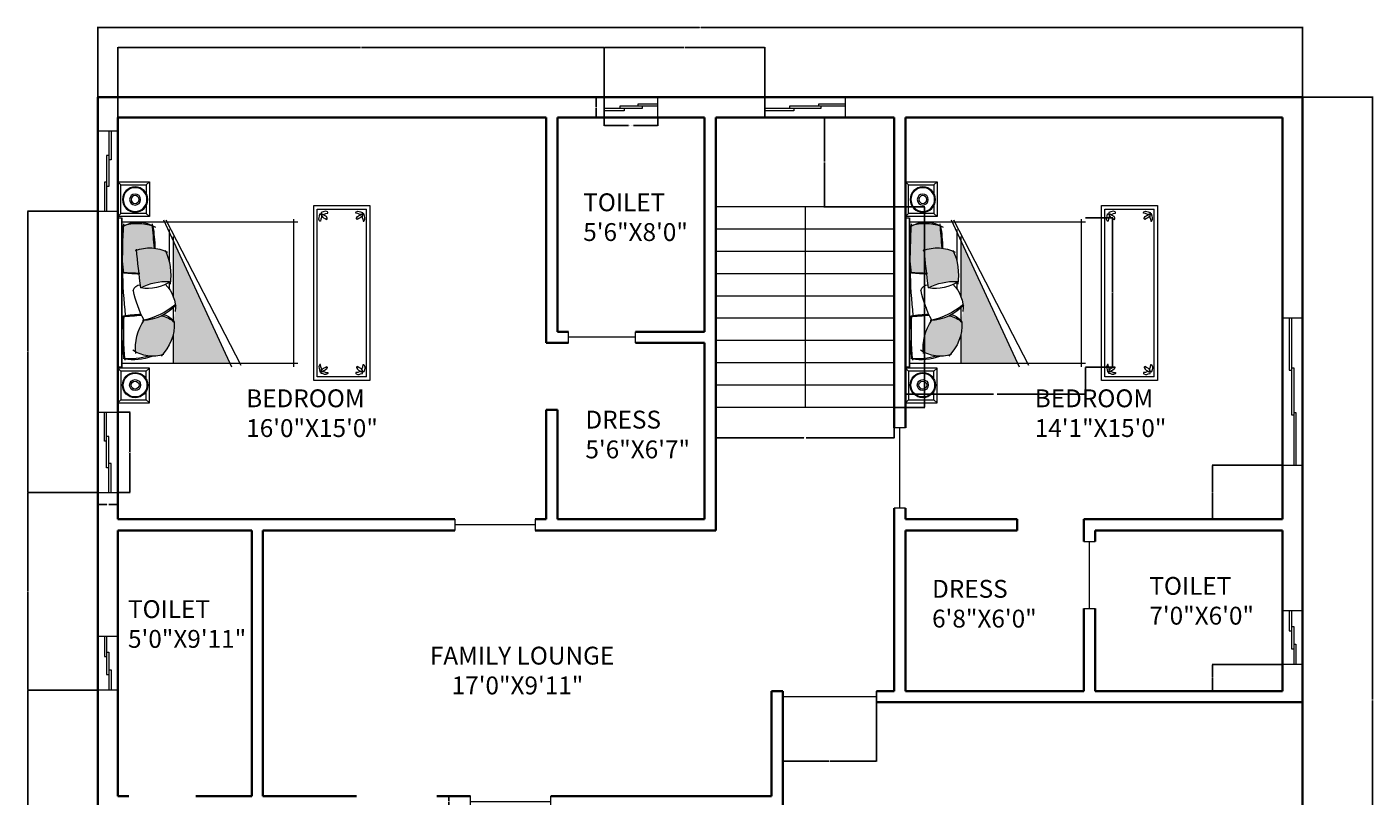
# Model space of a CAD drawing. Units: inches. Extents: x 1569 to 2779, y 1228 to 1844.
# Tile 6 of 6: x 2176 to 2779, y 1500 to 1844. Entities that reach past the tile are written whole.
import ezdxf

# ---------------------------------------------------------------- set-up
doc = ezdxf.new("R2010")
doc.units = ezdxf.units.IN
for name, color, linetype, lineweight in [('0.10', 252, 'Continuous', 9), ('0.15', 34, 'Continuous', 15), ('A-ANNO-DIMS', 2, 'Continuous', 18), ('A-AREA-IDEN', 7, 'Continuous', 18), ('A-DOOR', 3, 'Continuous', 20), ('A-FLOR-STRS', 4, 'Continuous', 18), ('A-FURN', 8, 'Continuous', 13), ('A-FURN-PATT', 116, 'Continuous', 9), ('A-GLAZ', 5, 'Continuous', 18), ('A-WALL', 7, 'Continuous', 35)]:
    doc.layers.add(name, color=color, linetype=linetype, lineweight=lineweight)
doc.styles.get("Standard").update_dxf_attribs({"font": 'arial.ttf'})
doc.dimstyles.get("Standard").update_dxf_attribs({"dimtxt": 0.18, "dimasz": 0.18, "dimexe": 0.18, "dimexo": 0.0625, "dimgap": 0.09, "dimtad": 0, "dimtih": 1, "dimtoh": 1, "dimdec": 4, "dimzin": 0, "dimdsep": 46, "dimtxsty": 'Standard', "dimcen": 0.09, "dimadec": 0, "dimazin": 0, "dimtfac": 1, "dimtdec": 4, "dimtofl": 0, "dimtmove": 0, "dimatfit": 3, "dimfxl": 1, "dimtolj": 1, "dimtzin": 0, "dimarcsym": 0})

# ---------------------------------------------------------------- blocks, each defined once
blk = doc.blocks.new('camita')
at = {"layer": '0.10'}
for p, q in [((-0.85, -0.045), (0.85, -0.045)), ((-0.805, -0.045), (-0.805, -2.048)), ((0.805, -0.045), (0.805, -2.048)), ((-0.827, -0.521), (0.846, -1.293)), ((-0.827, -0.548), (0.824, -1.399)), ((-0.716, -0.585), (-0.355, -0.585)), ((-0.114, -0.585), (-0.049, -0.585)), ((-0.638, -0.63), (0.043, -0.63)), ((0.175, -0.63), (0.318, -0.63)), ((0.474, -0.63), (0.805, -0.63)), ((-0.835, -2), (0.846, -2))]:
    blk.add_line(p, q, dxfattribs=at)
blk.add_lwpolyline([(-0.85, -0.041), (0.85, -0.041), (0.85, 0), (-0.85, 0)], close=True, dxfattribs=at)
for centre, radius, start, end in [((-0.457, -0.236), 0.344, 147.51, 213.8336), ((-0.2, -0.227), 0.586, 163.9263, 197.1409), ((-0.364, -5.846), 5.791, 83.8073, 94.1211), ((-0.51, -1.723), 1.678, 80.1255, 98.6619), ((2.353, -0.053), 2.58, 180.1063, 184.3854), ((-1.544, -0.245), 1.333, 359.9394, 7.5533), ((1.581, -0.289), 1.335, 170.3802, 178.9914), ((-1.44, -0.061), 1.712, 352.9291, 0.3959), ((0.452, -3.067), 3, 83.9026, 93.6759), ((0.486, -1.629), 1.578, 80.1602, 98.06), ((0.029, -0.138), 0.726, 342.5841, 6.0048), ((0.133, -0.17), 0.631, 339.923, 8.7433), ((-0.054, -0.363), 0.454, 159.3026, 206.5026), ((-1.33, -9.675), 9.499, 82.2708, 84.9399), ((0.458, -0.545), 0.584, 151.0456, 184.1497), ((-0.534, -0.339), 0.487, 327.2644, 9.0473), ((-0.007, -0.258), 0.0828, 100.018, 179.736), ((-0.293, -1.438), 1.29, 61.9749, 77.8435), ((-0.199, -0.274), 0.516, 310.7395, 359.0576), ((-0.567, -0.087), 0.906, 321.6953, 346.4626), ((0.627, -0.752), 0.551, 82.9691, 124.6739), ((0.32, -0.394), 0.404, 341.4524, 33.4512), ((-1.867, -14.986), 14.632, 84.6597, 85.7516), ((-0.46, 1.486), 1.909, 260.953, 268.6517), ((-0.2, 0.064), 0.667, 244.7809, 279.0606), ((0.179, -0.272), 0.383, 224.5284, 275.2229), ((0.438, -0.483), 0.19, 193.6849, 236.7035), ((0.571, -0.432), 0.315, 192.9388, 221.9636), ((0.361, -0.133), 0.51, 267.2589, 315.2997)]:
    blk.add_arc(centre, radius, start, end, dxfattribs=at)
blk = doc.blocks.new('VELADOR')
at = {"layer": '0.15'}
for p, q in [((-0.248, 0), (-0.203, -0.045)), ((0.248, 0), (0.202, -0.045)), ((-0.203, -0.405), (-0.248, -0.45)), ((0.248, -0.45), (0.202, -0.405))]:
    blk.add_line(p, q, dxfattribs=at)
blk.add_lwpolyline([(-0.248, 0), (-0.248, -0.45), (0.248, -0.45), (0.248, 0)], close=True, dxfattribs=at)
blk.add_lwpolyline([(0.092, -0.405), (0.202, -0.405), (0.202, -0.045), (-0.203, -0.045), (-0.203, -0.405), (-0.082, -0.405)], dxfattribs=at)
for radius in [0.18, 0.169, 0.0788, 0.0563]:
    blk.add_circle((0.005, -0.247), radius, dxfattribs=at)
blk = doc.blocks.new('carpet-7')
at = {"color": 0, "linetype": 'ByBlock'}
for p, q in [((-1.022, 0), (0, 0)), ((0, 0), (0, -0.54)), ((-1.694, -0.54), (-1.694, 0)), ((-1.694, 0), (-1.022, 0)), ((-1.658, -0.508), (-1.658, -0.032)), ((-1.658, -0.032), (-0.036, -0.032)), ((-1.636, -0.116), (-1.634, -0.103)), ((-1.629, -0.131), (-1.636, -0.116)), ((-1.634, -0.103), (-1.63, -0.09)), ((-1.63, -0.09), (-1.626, -0.07)), ((-1.626, -0.07), (-1.617, -0.069)), ((-1.617, -0.069), (-1.612, -0.072)), ((-1.615, -0.116), (-1.617, -0.134)), ((-1.608, -0.102), (-1.615, -0.116)), ((-1.611, -0.056), (-1.612, -0.064)), ((-1.612, -0.064), (-1.609, -0.068)), ((-1.612, -0.072), (-1.606, -0.089)), ((-1.59, -0.052), (-1.611, -0.056)), ((-1.609, -0.068), (-1.591, -0.073)), ((-1.609, -0.079), (-1.603, -0.072)), ((-1.599, -0.096), (-1.609, -0.079)), ((-1.606, -0.089), (-1.608, -0.102)), ((-1.603, -0.072), (-1.597, -0.072)), ((-1.593, -0.108), (-1.599, -0.096)), ((-1.597, -0.072), (-1.581, -0.081)), ((-1.585, -0.12), (-1.593, -0.108)), ((-1.591, -0.073), (-1.576, -0.072)), ((-1.575, -0.049), (-1.59, -0.052)), ((-1.569, -0.127), (-1.585, -0.12)), ((-1.581, -0.081), (-1.573, -0.092)), ((-1.576, -0.072), (-1.561, -0.066)), ((-1.561, -0.046), (-1.575, -0.049)), ((-1.573, -0.092), (-1.568, -0.107)), ((-1.563, -0.127), (-1.569, -0.127)), ((-1.568, -0.107), (-1.557, -0.123)), ((-1.557, -0.123), (-1.563, -0.127)), ((-1.544, -0.053), (-1.561, -0.046)), ((-1.561, -0.066), (-1.54, -0.064)), ((-1.54, -0.056), (-1.544, -0.053)), ((-1.54, -0.064), (-1.54, -0.056)), ((-0.151, -0.056), (-0.148, -0.053)), ((-0.151, -0.064), (-0.151, -0.056)), ((-0.131, -0.066), (-0.151, -0.064)), ((-0.148, -0.053), (-0.131, -0.046)), ((-0.124, -0.107), (-0.134, -0.123)), ((-0.134, -0.123), (-0.128, -0.127)), ((-0.131, -0.046), (-0.116, -0.049)), ((-0.115, -0.072), (-0.131, -0.066)), ((-0.128, -0.127), (-0.122, -0.127)), ((-0.119, -0.092), (-0.124, -0.107)), ((-0.122, -0.127), (-0.107, -0.12)), ((-0.11, -0.081), (-0.119, -0.092)), ((-0.116, -0.049), (-0.102, -0.052)), ((-0.101, -0.073), (-0.115, -0.072)), ((-0.095, -0.072), (-0.11, -0.081)), ((-0.107, -0.12), (-0.098, -0.108)), ((-0.102, -0.052), (-0.08, -0.056)), ((-0.083, -0.068), (-0.101, -0.073)), ((-0.098, -0.108), (-0.092, -0.096)), ((-0.089, -0.072), (-0.095, -0.072)), ((-0.092, -0.096), (-0.083, -0.079)), ((-0.083, -0.079), (-0.089, -0.072)), ((-0.079, -0.072), (-0.085, -0.089)), ((-0.085, -0.089), (-0.084, -0.102)), ((-0.084, -0.102), (-0.077, -0.116)), ((-0.079, -0.064), (-0.083, -0.068)), ((-0.08, -0.056), (-0.079, -0.064)), ((-0.074, -0.069), (-0.079, -0.072)), ((-0.077, -0.116), (-0.074, -0.134)), ((-0.066, -0.07), (-0.074, -0.069)), ((-0.061, -0.09), (-0.066, -0.07)), ((-0.062, -0.131), (-0.055, -0.116)), ((-0.058, -0.103), (-0.061, -0.09)), ((-0.055, -0.116), (-0.058, -0.103)), ((-0.036, -0.032), (-0.036, -0.508)), ((-1.626, -0.134), (-1.629, -0.131)), ((-1.617, -0.134), (-1.626, -0.134)), ((-0.074, -0.134), (-0.066, -0.134)), ((-0.066, -0.134), (-0.062, -0.131)), ((-1.658, -0.508), (-0.036, -0.508)), ((-1.629, -0.409), (-1.636, -0.424)), ((-1.636, -0.424), (-1.634, -0.437)), ((-1.634, -0.437), (-1.63, -0.45)), ((-1.63, -0.45), (-1.626, -0.47)), ((-1.626, -0.406), (-1.629, -0.409)), ((-1.617, -0.406), (-1.626, -0.406)), ((-1.626, -0.47), (-1.617, -0.471)), ((-1.615, -0.424), (-1.617, -0.406)), ((-1.617, -0.471), (-1.612, -0.468)), ((-1.608, -0.438), (-1.615, -0.424)), ((-1.612, -0.468), (-1.606, -0.451)), ((-1.612, -0.476), (-1.609, -0.472)), ((-1.611, -0.484), (-1.612, -0.476)), ((-1.59, -0.488), (-1.611, -0.484)), ((-1.599, -0.444), (-1.609, -0.461)), ((-1.609, -0.461), (-1.603, -0.468)), ((-1.609, -0.472), (-1.591, -0.467)), ((-1.606, -0.451), (-1.608, -0.438)), ((-1.603, -0.468), (-1.597, -0.468)), ((-1.593, -0.432), (-1.599, -0.444)), ((-1.597, -0.468), (-1.581, -0.459)), ((-1.585, -0.42), (-1.593, -0.432)), ((-1.591, -0.467), (-1.576, -0.468)), ((-1.575, -0.491), (-1.59, -0.488)), ((-1.569, -0.413), (-1.585, -0.42)), ((-1.581, -0.459), (-1.573, -0.448)), ((-1.576, -0.468), (-1.561, -0.474)), ((-1.561, -0.494), (-1.575, -0.491)), ((-1.573, -0.448), (-1.568, -0.433)), ((-1.563, -0.413), (-1.569, -0.413)), ((-1.568, -0.433), (-1.557, -0.417)), ((-1.557, -0.417), (-1.563, -0.413)), ((-1.561, -0.474), (-1.54, -0.476)), ((-1.544, -0.487), (-1.561, -0.494)), ((-1.54, -0.484), (-1.544, -0.487)), ((-1.54, -0.476), (-1.54, -0.484)), ((-0.131, -0.474), (-0.151, -0.476)), ((-0.151, -0.476), (-0.151, -0.484)), ((-0.151, -0.484), (-0.148, -0.487)), ((-0.148, -0.487), (-0.131, -0.494)), ((-0.134, -0.417), (-0.128, -0.413)), ((-0.124, -0.433), (-0.134, -0.417)), ((-0.115, -0.468), (-0.131, -0.474)), ((-0.131, -0.494), (-0.116, -0.491)), ((-0.128, -0.413), (-0.122, -0.413)), ((-0.119, -0.448), (-0.124, -0.433)), ((-0.122, -0.413), (-0.107, -0.42)), ((-0.11, -0.459), (-0.119, -0.448)), ((-0.116, -0.491), (-0.102, -0.488)), ((-0.101, -0.467), (-0.115, -0.468)), ((-0.095, -0.468), (-0.11, -0.459)), ((-0.107, -0.42), (-0.098, -0.432)), ((-0.102, -0.488), (-0.08, -0.484)), ((-0.083, -0.472), (-0.101, -0.467)), ((-0.098, -0.432), (-0.092, -0.444)), ((-0.089, -0.468), (-0.095, -0.468)), ((-0.092, -0.444), (-0.083, -0.461)), ((-0.083, -0.461), (-0.089, -0.468)), ((-0.085, -0.451), (-0.084, -0.438)), ((-0.079, -0.468), (-0.085, -0.451)), ((-0.084, -0.438), (-0.077, -0.424)), ((-0.079, -0.476), (-0.083, -0.472)), ((-0.08, -0.484), (-0.079, -0.476)), ((-0.074, -0.471), (-0.079, -0.468)), ((-0.077, -0.424), (-0.074, -0.406)), ((-0.074, -0.406), (-0.066, -0.406)), ((-0.066, -0.47), (-0.074, -0.471)), ((-0.066, -0.406), (-0.062, -0.409)), ((-0.061, -0.45), (-0.066, -0.47)), ((-0.062, -0.409), (-0.055, -0.424)), ((-0.058, -0.437), (-0.061, -0.45)), ((-0.055, -0.424), (-0.058, -0.437)), ((0, -0.54), (-1.694, -0.54))]:
    blk.add_line(p, q, dxfattribs=at)
blk = doc.blocks.new('WIN-24IN')
for p, q in [((9, 24), (0, 24)), ((3, 24), (3, 15)), ((4, 24), (4, 7)), ((3, 15), (4, 15)), ((4, 17), (5, 17)), ((5, 17), (5, 0)), ((4, 7), (5, 7)), ((5, 9), (6, 9)), ((6, 9), (6, 0)), ((9, 0), (0, 0))]:
    blk.add_line(p, q)
blk = doc.blocks.new('WIN-66IN')
for p, q in [((0, 0), (0, 9)), ((66, 0), (66, 9)), ((0, 4), (43.5, 4)), ((0, 3), (23.5, 3)), ((22.5, 5), (66, 5)), ((22.5, 4), (22.5, 5)), ((23.5, 3), (23.5, 4)), ((42.5, 6), (66, 6)), ((42.5, 5), (42.5, 6)), ((43.5, 4), (43.5, 5))]:
    blk.add_line(p, q)
blk = doc.blocks.new('WIN-36IN-A')
for p, q in [((0, 9), (0, 0)), ((36, 9), (36, 0)), ((25, 4), (0, 4)), ((13, 3), (0, 3)), ((36, 5), (11, 5)), ((11, 5), (11, 4)), ((13, 4), (13, 3)), ((24, 6), (24, 5)), ((36, 6), (24, 6)), ((25, 5), (25, 4))]:
    blk.add_line(p, q)
blk = doc.blocks.new('WIN-36IN-B')
for p, q in [((0, 36), (9, 36)), ((3, 23), (3, 36)), ((4, 11), (4, 36)), ((5, 25), (4, 25)), ((5, 0), (5, 25)), ((4, 23), (3, 23)), ((6, 13), (5, 13)), ((6, 0), (6, 13)), ((5, 11), (4, 11)), ((0, 0), (9, 0))]:
    blk.add_line(p, q)
blk = doc.blocks.new('DOOR-30IN')
for p, q in [((0, 5), (0, 0)), ((0, 2.5), (30, 2.5)), ((30, 5), (30, 0))]:
    blk.add_line(p, q)
blk = doc.blocks.new('DOOR-36IN')
for p, q in [((0, 5), (0, 0)), ((36, 2.5), (0, 2.5)), ((36, 5), (36, 0))]:
    blk.add_line(p, q)
blk = doc.blocks.new('STAIR-RETURN-FLIGHT')
for p, q in [((80, 90), (0, 90)), ((40, 90), (40, 0)), ((80, 80), (0, 80)), ((80, 70), (0, 70)), ((80, 60), (0, 60)), ((80, 50), (0, 50)), ((80, 40), (0, 40)), ((80, 30), (0, 30)), ((80, 20), (0, 20)), ((80, 10), (0, 10)), ((80, 0), (0, 0))]:
    blk.add_line(p, q)
blk = doc.blocks.new('*D22')
at = {"layer": 'A-ANNO-DIMS', "color": 0, "lineweight": -2, "transparency": 16777216}
for p, q in [((2359.41, 1499.88), (2364.93, 1499.88)), ((2364.75, 1499.7), (2364.75, 1497.56)), ((2364.75, 1495.06), (2364.75, 1497.2)), ((2359.41, 1494.88), (2364.93, 1494.88))]:
    blk.add_line(p, q, dxfattribs=at)
at = {"layer": 'A-ANNO-DIMS', "color": 0, "transparency": 16777216}
for points in [[(2364.72, 1499.7), (2364.78, 1499.7), (2364.75, 1499.88)], [(2364.72, 1495.06), (2364.78, 1495.06), (2364.75, 1494.88)]]:
    blk.add_solid(points, dxfattribs=at)
at = {"layer": 'Defpoints', "color": 0, "transparency": 16777216}
for p in [(2359.35, 1499.88), (2364.75, 1499.88), (2359.35, 1494.88)]:
    blk.add_point(p, dxfattribs=at)
at = {"layer": 'A-ANNO-DIMS', "color": 0, "transparency": 16777216, "insert": (2364.75, 1497.38), "char_height": 0.18, "attachment_point": 5}
blk.add_mtext('\\A1;5 TYP.', dxfattribs=at)
blk = doc.blocks.new('*D23')
at = {"layer": 'A-ANNO-DIMS', "color": 0, "lineweight": -2, "transparency": 16777216}
for p, q in [((2434.35, 1803.82), (2434.35, 1800.1)), ((2458.35, 1803.82), (2458.35, 1800.1)), ((2434.53, 1800.28), (2445.23, 1800.28)), ((2458.17, 1800.28), (2447.47, 1800.28))]:
    blk.add_line(p, q, dxfattribs=at)
at = {"layer": 'A-ANNO-DIMS', "color": 0, "transparency": 16777216}
for points in [[(2434.53, 1800.31), (2434.53, 1800.25), (2434.35, 1800.28)], [(2458.17, 1800.31), (2458.17, 1800.25), (2458.35, 1800.28)]]:
    blk.add_solid(points, dxfattribs=at)
at = {"layer": 'Defpoints', "color": 0, "transparency": 16777216}
for p in [(2434.35, 1803.88), (2458.35, 1803.88), (2458.35, 1800.28)]:
    blk.add_point(p, dxfattribs=at)
at = {"layer": 'A-ANNO-DIMS', "color": 0, "transparency": 16777216, "insert": (2446.35, 1800.28), "char_height": 0.18, "attachment_point": 5}
blk.add_mtext('\\A1;WINDOW 24 TYP.', dxfattribs=at)
blk = doc.blocks.new('*D24')
at = {"layer": 'A-ANNO-DIMS', "color": 0, "lineweight": -2, "transparency": 16777216}
for p, q in [((2434.29, 1812.88), (2430.57, 1812.88)), ((2430.75, 1812.7), (2430.75, 1808.56)), ((2434.29, 1803.88), (2430.57, 1803.88)), ((2430.75, 1804.06), (2430.75, 1808.2))]:
    blk.add_line(p, q, dxfattribs=at)
at = {"layer": 'A-ANNO-DIMS', "color": 0, "transparency": 16777216}
for points in [[(2430.72, 1812.7), (2430.78, 1812.7), (2430.75, 1812.88)], [(2430.72, 1804.06), (2430.78, 1804.06), (2430.75, 1803.88)]]:
    blk.add_solid(points, dxfattribs=at)
at = {"layer": 'Defpoints', "color": 0, "transparency": 16777216}
for p in [(2434.35, 1812.88), (2430.75, 1803.88), (2434.35, 1803.88)]:
    blk.add_point(p, dxfattribs=at)
at = {"layer": 'A-ANNO-DIMS', "color": 0, "transparency": 16777216, "insert": (2430.75, 1808.38), "char_height": 0.18, "attachment_point": 5}
blk.add_mtext('\\A1;9 TYP.', dxfattribs=at)
blk = doc.blocks.new('*D27')
at = {"layer": 'A-ANNO-DIMS', "color": 0, "lineweight": -2, "transparency": 16777216}
for p, q in [((2216.41, 1671.88), (2221.93, 1671.88)), ((2221.75, 1671.7), (2221.75, 1654.06)), ((2221.75, 1636.06), (2221.75, 1653.7)), ((2216.41, 1635.88), (2221.93, 1635.88))]:
    blk.add_line(p, q, dxfattribs=at)
at = {"layer": 'A-ANNO-DIMS', "color": 0, "transparency": 16777216}
for points in [[(2221.72, 1671.7), (2221.78, 1671.7), (2221.75, 1671.88)], [(2221.72, 1636.06), (2221.78, 1636.06), (2221.75, 1635.88)]]:
    blk.add_solid(points, dxfattribs=at)
at = {"layer": 'Defpoints', "color": 0, "transparency": 16777216}
for p in [(2216.35, 1671.88), (2221.75, 1671.88), (2216.35, 1635.88)]:
    blk.add_point(p, dxfattribs=at)
at = {"layer": 'A-ANNO-DIMS', "color": 0, "transparency": 16777216, "insert": (2221.75, 1653.88), "char_height": 0.18, "attachment_point": 5}
blk.add_mtext('\\A1;WINDOW 36 TYP.', dxfattribs=at)
blk = doc.blocks.new('*D28')
at = {"layer": 'A-ANNO-DIMS', "color": 0, "lineweight": -2, "transparency": 16777216}
for p, q in [((2207.35, 1635.82), (2207.35, 1630.3)), ((2216.35, 1635.82), (2216.35, 1630.3)), ((2207.53, 1630.48), (2211.39, 1630.48)), ((2216.17, 1630.48), (2212.31, 1630.48))]:
    blk.add_line(p, q, dxfattribs=at)
at = {"layer": 'A-ANNO-DIMS', "color": 0, "transparency": 16777216}
for points in [[(2207.53, 1630.51), (2207.53, 1630.45), (2207.35, 1630.48)], [(2216.17, 1630.51), (2216.17, 1630.45), (2216.35, 1630.48)]]:
    blk.add_solid(points, dxfattribs=at)
at = {"layer": 'Defpoints', "color": 0, "transparency": 16777216}
for p in [(2207.35, 1635.88), (2216.35, 1635.88), (2216.35, 1630.48)]:
    blk.add_point(p, dxfattribs=at)
at = {"layer": 'A-ANNO-DIMS', "color": 0, "transparency": 16777216, "insert": (2211.85, 1630.48), "char_height": 0.18, "attachment_point": 5}
blk.add_mtext('\\A1;9 TYP.', dxfattribs=at)
blk = doc.blocks.new('*D31')
at = {"layer": 'A-ANNO-DIMS', "color": 0, "lineweight": -2, "transparency": 16777216}
for p, q in [((2569.35, 1691.89), (2569.35, 1679.67)), ((2650.01, 1691.89), (2650.01, 1679.67)), ((2569.53, 1679.85), (2608.86, 1679.85)), ((2649.83, 1679.85), (2610.5, 1679.85))]:
    blk.add_line(p, q, dxfattribs=at)
at = {"layer": 'A-ANNO-DIMS', "color": 0, "transparency": 16777216}
for points in [[(2569.53, 1679.88), (2569.53, 1679.82), (2569.35, 1679.85)], [(2649.83, 1679.88), (2649.83, 1679.82), (2650.01, 1679.85)]]:
    blk.add_solid(points, dxfattribs=at)
at = {"layer": 'Defpoints', "color": 0, "transparency": 16777216}
for p in [(2569.35, 1691.95), (2650.01, 1691.95), (2569.35, 1679.85)]:
    blk.add_point(p, dxfattribs=at)
at = {"layer": 'A-ANNO-DIMS', "color": 0, "transparency": 16777216, "insert": (2609.68, 1679.85), "char_height": 0.18, "attachment_point": 5}
blk.add_mtext('\\A1;BED 81 TYP.', dxfattribs=at)
blk = doc.blocks.new('*D32')
at = {"layer": 'A-ANNO-DIMS', "color": 0, "lineweight": -2, "transparency": 16777216}
for p, q in [((2650.07, 1758.89), (2662.29, 1758.89)), ((2662.11, 1758.71), (2662.11, 1725.6)), ((2662.11, 1692.13), (2662.11, 1725.24)), ((2650.07, 1691.95), (2662.29, 1691.95))]:
    blk.add_line(p, q, dxfattribs=at)
at = {"layer": 'A-ANNO-DIMS', "color": 0, "transparency": 16777216}
for points in [[(2662.08, 1758.71), (2662.14, 1758.71), (2662.11, 1758.89)], [(2662.08, 1692.13), (2662.14, 1692.13), (2662.11, 1691.95)]]:
    blk.add_solid(points, dxfattribs=at)
at = {"layer": 'Defpoints', "color": 0, "transparency": 16777216}
for p in [(2650.01, 1758.89), (2650.01, 1691.95), (2662.11, 1691.95)]:
    blk.add_point(p, dxfattribs=at)
at = {"layer": 'A-ANNO-DIMS', "color": 0, "transparency": 16777216, "insert": (2662.11, 1725.42), "char_height": 0.18, "attachment_point": 5}
blk.add_mtext('\\A1;67 TYP.', dxfattribs=at)
blk = doc.blocks.new('*D37')
at = {"layer": 'A-ANNO-DIMS', "color": 0, "lineweight": -2, "transparency": 16777216}
for p, q in [((2564.41, 1763.88), (2578.03, 1763.88)), ((2577.85, 1763.7), (2577.85, 1719.06)), ((2577.85, 1674.06), (2577.85, 1718.7)), ((2564.41, 1673.88), (2578.03, 1673.88))]:
    blk.add_line(p, q, dxfattribs=at)
at = {"layer": 'A-ANNO-DIMS', "color": 0, "transparency": 16777216}
for points in [[(2577.82, 1763.7), (2577.88, 1763.7), (2577.85, 1763.88)], [(2577.82, 1674.06), (2577.88, 1674.06), (2577.85, 1673.88)]]:
    blk.add_solid(points, dxfattribs=at)
at = {"layer": 'Defpoints', "color": 0, "transparency": 16777216}
for p in [(2564.35, 1763.88), (2577.85, 1763.88), (2564.35, 1673.88)]:
    blk.add_point(p, dxfattribs=at)
at = {"layer": 'A-ANNO-DIMS', "color": 0, "transparency": 16777216, "insert": (2577.85, 1718.88), "char_height": 0.18, "attachment_point": 5}
blk.add_mtext('\\A1;STAIR FLIGHT 90 TYP.', dxfattribs=at)
blk = doc.blocks.new('*D38')
at = {"layer": 'A-ANNO-DIMS', "color": 0, "lineweight": -2, "transparency": 16777216}
for p, q in [((2484.35, 1673.82), (2484.35, 1660.2)), ((2564.35, 1673.82), (2564.35, 1660.2)), ((2484.53, 1660.38), (2523.82, 1660.38)), ((2564.17, 1660.38), (2524.88, 1660.38))]:
    blk.add_line(p, q, dxfattribs=at)
at = {"layer": 'A-ANNO-DIMS', "color": 0, "transparency": 16777216}
for points in [[(2484.53, 1660.41), (2484.53, 1660.35), (2484.35, 1660.38)], [(2564.17, 1660.41), (2564.17, 1660.35), (2564.35, 1660.38)]]:
    blk.add_solid(points, dxfattribs=at)
at = {"layer": 'Defpoints', "color": 0, "transparency": 16777216}
for p in [(2484.35, 1673.88), (2564.35, 1673.88), (2564.35, 1660.38)]:
    blk.add_point(p, dxfattribs=at)
at = {"layer": 'A-ANNO-DIMS', "color": 0, "transparency": 16777216, "insert": (2524.35, 1660.38), "char_height": 0.18, "attachment_point": 5}
blk.add_mtext('\\A1;80 TYP.', dxfattribs=at)
blk = doc.blocks.new('*D50')
at = {"layer": 'A-ANNO-DIMS', "color": 0, "lineweight": -2, "transparency": 16777216}
for p, q in [((2207.35, 1812.94), (2207.35, 1844.41)), ((2207.53, 1844.23), (2477.06, 1844.23)), ((2747.17, 1844.23), (2477.64, 1844.23)), ((2747.35, 1812.94), (2747.35, 1844.41))]:
    blk.add_line(p, q, dxfattribs=at)
at = {"layer": 'A-ANNO-DIMS', "color": 0, "transparency": 16777216}
for points in [[(2207.53, 1844.26), (2207.53, 1844.2), (2207.35, 1844.23)], [(2747.17, 1844.26), (2747.17, 1844.2), (2747.35, 1844.23)]]:
    blk.add_solid(points, dxfattribs=at)
at = {"layer": 'Defpoints', "color": 0, "transparency": 16777216}
for p in [(2747.35, 1844.23), (2207.35, 1812.88), (2747.35, 1812.88)]:
    blk.add_point(p, dxfattribs=at)
at = {"layer": 'A-ANNO-DIMS', "color": 0, "transparency": 16777216, "insert": (2477.35, 1844.23), "char_height": 0.18, "attachment_point": 5}
blk.add_mtext('\\A1;540', dxfattribs=at)
blk = doc.blocks.new('*D51')
at = {"layer": 'A-ANNO-DIMS', "color": 0, "lineweight": -2, "transparency": 16777216}
for p, q in [((2747.41, 1812.88), (2778.88, 1812.88)), ((2778.7, 1812.7), (2778.7, 1543.06)), ((2778.7, 1273.06), (2778.7, 1542.7)), ((2747.41, 1272.88), (2778.88, 1272.88))]:
    blk.add_line(p, q, dxfattribs=at)
at = {"layer": 'A-ANNO-DIMS', "color": 0, "transparency": 16777216}
for points in [[(2778.67, 1812.7), (2778.73, 1812.7), (2778.7, 1812.88)], [(2778.67, 1273.06), (2778.73, 1273.06), (2778.7, 1272.88)]]:
    blk.add_solid(points, dxfattribs=at)
at = {"layer": 'Defpoints', "color": 0, "transparency": 16777216}
for p in [(2747.35, 1812.88), (2778.7, 1812.88), (2747.35, 1272.88)]:
    blk.add_point(p, dxfattribs=at)
at = {"layer": 'A-ANNO-DIMS', "color": 0, "transparency": 16777216, "insert": (2778.7, 1542.88), "char_height": 0.18, "attachment_point": 5}
blk.add_mtext('\\A1;540', dxfattribs=at)
blk = doc.blocks.new('*D69')
at = {"layer": 'A-ANNO-DIMS', "color": 0, "lineweight": -2, "transparency": 16777216}
for p, q in [((2216.35, 1803.94), (2216.35, 1835.41)), ((2216.53, 1835.23), (2325.06, 1835.23)), ((2434.17, 1835.23), (2325.64, 1835.23)), ((2434.35, 1803.94), (2434.35, 1835.41))]:
    blk.add_line(p, q, dxfattribs=at)
at = {"layer": 'A-ANNO-DIMS', "color": 0, "transparency": 16777216}
for points in [[(2216.53, 1835.26), (2216.53, 1835.2), (2216.35, 1835.23)], [(2434.17, 1835.26), (2434.17, 1835.2), (2434.35, 1835.23)]]:
    blk.add_solid(points, dxfattribs=at)
at = {"layer": 'Defpoints', "color": 0, "transparency": 16777216}
for p in [(2434.35, 1835.23), (2216.35, 1803.88), (2434.35, 1803.88)]:
    blk.add_point(p, dxfattribs=at)
at = {"layer": 'A-ANNO-DIMS', "color": 0, "transparency": 16777216, "insert": (2325.35, 1835.23), "char_height": 0.18, "attachment_point": 5}
blk.add_mtext('\\A1;218', dxfattribs=at)
blk = doc.blocks.new('*D70')
at = {"layer": 'A-ANNO-DIMS', "color": 0, "lineweight": -2, "transparency": 16777216}
for p, q in [((2434.35, 1803.94), (2434.35, 1835.41)), ((2434.53, 1835.23), (2470.13, 1835.23)), ((2506.17, 1835.23), (2470.57, 1835.23)), ((2506.35, 1803.94), (2506.35, 1835.41))]:
    blk.add_line(p, q, dxfattribs=at)
at = {"layer": 'A-ANNO-DIMS', "color": 0, "transparency": 16777216}
for points in [[(2434.53, 1835.26), (2434.53, 1835.2), (2434.35, 1835.23)], [(2506.17, 1835.26), (2506.17, 1835.2), (2506.35, 1835.23)]]:
    blk.add_solid(points, dxfattribs=at)
at = {"layer": 'Defpoints', "color": 0, "transparency": 16777216}
for p in [(2506.35, 1835.23), (2434.35, 1803.88), (2506.35, 1803.88)]:
    blk.add_point(p, dxfattribs=at)
at = {"layer": 'A-ANNO-DIMS', "color": 0, "transparency": 16777216, "insert": (2470.35, 1835.23), "char_height": 0.18, "attachment_point": 5}
blk.add_mtext('\\A1;72', dxfattribs=at)
blk = doc.blocks.new('*D74')
at = {"layer": 'A-ANNO-DIMS', "color": 0, "lineweight": -2, "transparency": 16777216}
for p, q in [((2207.29, 1547.38), (2175.82, 1547.38)), ((2176, 1547.2), (2176, 1472.5)), ((2176, 1397.43), (2176, 1472.13)), ((2207.29, 1397.25), (2175.82, 1397.25))]:
    blk.add_line(p, q, dxfattribs=at)
at = {"layer": 'A-ANNO-DIMS', "color": 0, "transparency": 16777216}
for points in [[(2175.97, 1547.2), (2176.03, 1547.2), (2176, 1547.38)], [(2175.97, 1397.43), (2176.03, 1397.43), (2176, 1397.25)]]:
    blk.add_solid(points, dxfattribs=at)
at = {"layer": 'Defpoints', "color": 0, "transparency": 16777216}
for p in [(2176, 1547.38), (2207.35, 1547.38), (2207.35, 1397.25)]:
    blk.add_point(p, dxfattribs=at)
at = {"layer": 'A-ANNO-DIMS', "color": 0, "transparency": 16777216, "insert": (2176, 1472.31), "char_height": 0.18, "attachment_point": 5}
blk.add_mtext('\\A1;150.13', dxfattribs=at)
blk = doc.blocks.new('*D75')
at = {"layer": 'A-ANNO-DIMS', "color": 0, "lineweight": -2, "transparency": 16777216}
for p, q in [((2207.29, 1635.88), (2175.82, 1635.88)), ((2176, 1635.7), (2176, 1591.81)), ((2176, 1547.56), (2176, 1591.45)), ((2207.29, 1547.38), (2175.82, 1547.38))]:
    blk.add_line(p, q, dxfattribs=at)
at = {"layer": 'A-ANNO-DIMS', "color": 0, "transparency": 16777216}
for points in [[(2175.97, 1635.7), (2176.03, 1635.7), (2176, 1635.88)], [(2175.97, 1547.56), (2176.03, 1547.56), (2176, 1547.38)]]:
    blk.add_solid(points, dxfattribs=at)
at = {"layer": 'Defpoints', "color": 0, "transparency": 16777216}
for p in [(2176, 1635.88), (2207.35, 1635.88), (2207.35, 1547.38)]:
    blk.add_point(p, dxfattribs=at)
at = {"layer": 'A-ANNO-DIMS', "color": 0, "transparency": 16777216, "insert": (2176, 1591.63), "char_height": 0.18, "attachment_point": 5}
blk.add_mtext('\\A1;88.5', dxfattribs=at)
blk = doc.blocks.new('*D76')
at = {"layer": 'A-ANNO-DIMS', "color": 0, "lineweight": -2, "transparency": 16777216}
for p, q in [((2207.29, 1761.88), (2175.82, 1761.88)), ((2176, 1761.7), (2176, 1699.06)), ((2176, 1636.06), (2176, 1698.7)), ((2207.29, 1635.88), (2175.82, 1635.88))]:
    blk.add_line(p, q, dxfattribs=at)
at = {"layer": 'A-ANNO-DIMS', "color": 0, "transparency": 16777216}
for points in [[(2175.97, 1761.7), (2176.03, 1761.7), (2176, 1761.88)], [(2175.97, 1636.06), (2176.03, 1636.06), (2176, 1635.88)]]:
    blk.add_solid(points, dxfattribs=at)
at = {"layer": 'Defpoints', "color": 0, "transparency": 16777216}
for p in [(2176, 1761.88), (2207.35, 1761.88), (2207.35, 1635.88)]:
    blk.add_point(p, dxfattribs=at)
at = {"layer": 'A-ANNO-DIMS', "color": 0, "transparency": 16777216, "insert": (2176, 1698.88), "char_height": 0.18, "attachment_point": 5}
blk.add_mtext('\\A1;126', dxfattribs=at)
blk = doc.blocks.new('*D77')
at = {"layer": 'A-ANNO-DIMS', "color": 0, "lineweight": -2, "transparency": 16777216}
for p, q in [((2738.29, 1558.88), (2706.82, 1558.88)), ((2707, 1558.7), (2707, 1553.06)), ((2707, 1547.06), (2707, 1552.7)), ((2738.29, 1546.88), (2706.82, 1546.88))]:
    blk.add_line(p, q, dxfattribs=at)
at = {"layer": 'A-ANNO-DIMS', "color": 0, "transparency": 16777216}
for points in [[(2706.97, 1558.7), (2707.03, 1558.7), (2707, 1558.88)], [(2706.97, 1547.06), (2707.03, 1547.06), (2707, 1546.88)]]:
    blk.add_solid(points, dxfattribs=at)
at = {"layer": 'Defpoints', "color": 0, "transparency": 16777216}
for p in [(2707, 1558.88), (2738.35, 1558.88), (2738.35, 1546.88)]:
    blk.add_point(p, dxfattribs=at)
at = {"layer": 'A-ANNO-DIMS', "color": 0, "transparency": 16777216, "insert": (2707, 1552.88), "char_height": 0.18, "attachment_point": 5}
blk.add_mtext('\\A1;12', dxfattribs=at)
blk = doc.blocks.new('*D78')
at = {"layer": 'A-ANNO-DIMS', "color": 0, "lineweight": -2, "transparency": 16777216}
for p, q in [((2738.29, 1648.14), (2706.82, 1648.14)), ((2707, 1647.96), (2707, 1636.19)), ((2707, 1624.06), (2707, 1635.83)), ((2738.29, 1623.88), (2706.82, 1623.88))]:
    blk.add_line(p, q, dxfattribs=at)
at = {"layer": 'A-ANNO-DIMS', "color": 0, "transparency": 16777216}
for points in [[(2706.97, 1647.96), (2707.03, 1647.96), (2707, 1648.14)], [(2706.97, 1624.06), (2707.03, 1624.06), (2707, 1623.88)]]:
    blk.add_solid(points, dxfattribs=at)
at = {"layer": 'Defpoints', "color": 0, "transparency": 16777216}
for p in [(2707, 1648.14), (2738.35, 1648.14), (2738.35, 1623.88)]:
    blk.add_point(p, dxfattribs=at)
at = {"layer": 'A-ANNO-DIMS', "color": 0, "transparency": 16777216, "insert": (2707, 1636.01), "char_height": 0.18, "attachment_point": 5}
blk.add_mtext('\\A1;24.264', dxfattribs=at)
blk = doc.blocks.new('*D79')
at = {"layer": 'A-ANNO-DIMS', "color": 0, "lineweight": -2, "transparency": 16777216}
for p, q in [((2564.29, 1803.88), (2532.82, 1803.88)), ((2533, 1803.7), (2533, 1784.06)), ((2533, 1764.06), (2533, 1783.7)), ((2564.29, 1763.88), (2532.82, 1763.88))]:
    blk.add_line(p, q, dxfattribs=at)
at = {"layer": 'A-ANNO-DIMS', "color": 0, "transparency": 16777216}
for points in [[(2532.97, 1803.7), (2533.03, 1803.7), (2533, 1803.88)], [(2532.97, 1764.06), (2533.03, 1764.06), (2533, 1763.88)]]:
    blk.add_solid(points, dxfattribs=at)
at = {"layer": 'Defpoints', "color": 0, "transparency": 16777216}
for p in [(2533, 1803.88), (2564.35, 1803.88), (2564.35, 1763.88)]:
    blk.add_point(p, dxfattribs=at)
at = {"layer": 'A-ANNO-DIMS', "color": 0, "transparency": 16777216, "insert": (2533, 1783.88), "char_height": 0.18, "attachment_point": 5}
blk.add_mtext('\\A1;40', dxfattribs=at)
blk = doc.blocks.new('*D83')
at = {"layer": 'A-ANNO-DIMS', "color": 0, "lineweight": -2, "transparency": 16777216}
for p, q in [((2514.35, 1546.82), (2514.35, 1515.35)), ((2556.35, 1546.82), (2556.35, 1515.35)), ((2514.53, 1515.53), (2535.13, 1515.53)), ((2556.17, 1515.53), (2535.57, 1515.53))]:
    blk.add_line(p, q, dxfattribs=at)
at = {"layer": 'A-ANNO-DIMS', "color": 0, "transparency": 16777216}
for points in [[(2514.53, 1515.56), (2514.53, 1515.5), (2514.35, 1515.53)], [(2556.17, 1515.56), (2556.17, 1515.5), (2556.35, 1515.53)]]:
    blk.add_solid(points, dxfattribs=at)
at = {"layer": 'Defpoints', "color": 0, "transparency": 16777216}
for p in [(2514.35, 1546.88), (2556.35, 1546.88), (2514.35, 1515.53)]:
    blk.add_point(p, dxfattribs=at)
at = {"layer": 'A-ANNO-DIMS', "color": 0, "transparency": 16777216, "insert": (2535.35, 1515.53), "char_height": 0.18, "attachment_point": 5}
blk.add_mtext('\\A1;42', dxfattribs=at)

msp = doc.modelspace()

# ---------------------------------------------------------------- hatches: boundary and pattern name
at = {"layer": 'A-FURN-PATT'}
h = msp.add_hatch(color=256, dxfattribs=at)
h.dxf.hatch_style = 1
h.paths.add_polyline_path([(2231.9265, 1755.3888, 0.14222248), (2219.0532, 1755.5152, 0.02322168), (2218.5711, 1734.3523, -0.01794435), (2225.8563, 1734.0816, -0.00696723), (2224.7826, 1744.4488, -0.11389129), (2232.7792, 1745.3149, -0.00438694)])
h.paths.add_polyline_path([(2241.1575, 1723.7086, -0.16677621), (2241.4673, 1713.9309, -0.09017801), (2241.1575, 1706.7575), (2241.1575, 1693.7212), (2266.5173, 1693.7212), (2241.1575, 1748.683)])
h = msp.add_hatch(color=256, dxfattribs=at)
h.dxf.hatch_style = 1
h.paths.add_polyline_path([(2584.9265, 1755.3888, 0.14222248), (2572.0532, 1755.5152, 0.02322168), (2571.5711, 1734.3523, -0.01794435), (2578.8563, 1734.0816, -0.00696723), (2577.7826, 1744.4488, -0.11389129), (2585.7792, 1745.3149, -0.00438694)])
h.paths.add_polyline_path([(2594.1575, 1723.7086, -0.16677621), (2594.4673, 1713.9309, -0.09017801), (2594.1575, 1706.7575), (2594.1575, 1693.7212), (2619.5173, 1693.7212), (2594.1575, 1748.683)])
h = msp.add_hatch(color=256, dxfattribs=at)
h.dxf.hatch_style = 1
h.paths.add_polyline_path([(2237.8675, 1743.9727, 0.18953567), (2224.7889, 1744.4952, 0.01140771), (2226.6975, 1727.5384, -0.1503613), (2239.9372, 1730.3169, 0.13377603)])
h.paths.add_polyline_path([(2224.363, 1698.8217, 0.1949524), (2236.255, 1697.541, 0.20255928), (2241.6379, 1712.2024, 0.12732633), (2236.1303, 1715.0635, -0.10404536), (2228.0277, 1712.9922, 0.17383481)])
h = msp.add_hatch(color=256, dxfattribs=at)
h.dxf.hatch_style = 1
h.paths.add_polyline_path([(2590.8675, 1743.9727, 0.18953567), (2577.7889, 1744.4952, 0.01140771), (2579.6975, 1727.5384, -0.1503613), (2592.9372, 1730.3169, 0.13377603)])
h.paths.add_polyline_path([(2577.363, 1698.8217, 0.1949524), (2589.255, 1697.541, 0.20255928), (2594.6379, 1712.2024, 0.12732633), (2589.1303, 1715.0635, -0.10404536), (2581.0277, 1712.9922, 0.17383481)])

# ---------------------------------------------------------------- linework, layer by layer
at = {"layer": 'A-DOOR'}
for p, q in [((2556.3512, 1541.8785), (2556.3512, 1546.8785)), ((2556.3512, 1544.3785), (2514.3512, 1544.3785))]:
    msp.add_line(p, q, dxfattribs=at)
at = {"layer": 'A-WALL'}
for p, q in [((2747.3512, 1812.8785), (2207.3512, 1812.8785)), ((2207.3512, 1812.8785), (2207.3512, 1272.8785)), ((2747.3512, 1272.8785), (2747.3512, 1812.8785)), ((2408.3512, 1803.8785), (2216.3512, 1803.8785)), ((2216.3512, 1803.8785), (2216.3512, 1623.8785)), ((2408.3512, 1803.8785), (2408.3512, 1702.8785)), ((2479.3512, 1803.8785), (2413.3512, 1803.8785)), ((2413.3512, 1803.8785), (2413.3512, 1707.8785)), ((2479.3512, 1803.8785), (2479.3512, 1707.8785)), ((2564.3512, 1803.8785), (2484.3512, 1803.8785)), ((2484.3512, 1803.8785), (2484.3512, 1618.8785)), ((2564.3512, 1664.8785), (2564.3512, 1803.8785)), ((2569.3512, 1664.8785), (2569.3512, 1803.8785)), ((2738.3512, 1803.8785), (2569.3512, 1803.8785)), ((2738.3512, 1623.8785), (2738.3512, 1803.8785)), ((2418.3512, 1707.8785), (2413.3512, 1707.8785)), ((2479.3512, 1707.8785), (2448.3512, 1707.8785)), ((2418.3512, 1702.8785), (2408.3512, 1702.8785)), ((2479.3512, 1702.8785), (2448.3512, 1702.8785)), ((2479.3512, 1702.8785), (2479.3512, 1623.8785)), ((2413.3512, 1672.8785), (2408.3512, 1672.8785)), ((2408.3512, 1672.8785), (2408.3512, 1623.8785)), ((2413.3512, 1672.8785), (2413.3512, 1623.8785)), ((2564.3512, 1546.8785), (2564.3512, 1628.8785)), ((2569.3512, 1623.8785), (2569.3512, 1628.8785)), ((2367.3512, 1623.8785), (2216.3512, 1623.8785)), ((2408.3512, 1623.8785), (2403.3512, 1623.8785)), ((2479.3512, 1623.8785), (2413.3512, 1623.8785)), ((2619.3512, 1623.8785), (2569.3512, 1623.8785)), ((2619.3512, 1618.8785), (2619.3512, 1623.8785)), ((2738.3512, 1623.8785), (2649.3512, 1623.8785)), ((2649.3512, 1613.8785), (2649.3512, 1623.8785)), ((2216.3512, 1618.8785), (2216.3512, 1499.8785)), ((2276.3512, 1618.8785), (2216.3512, 1618.8785)), ((2276.3512, 1618.8785), (2276.3512, 1499.8785)), ((2367.3512, 1618.8785), (2281.3512, 1618.8785)), ((2281.3512, 1618.8785), (2281.3512, 1499.8785)), ((2484.3512, 1618.8785), (2403.3512, 1618.8785)), ((2569.3512, 1546.8785), (2569.3512, 1618.8785)), ((2619.3512, 1618.8785), (2569.3512, 1618.8785)), ((2738.3512, 1618.8785), (2654.3512, 1618.8785)), ((2654.3512, 1613.8785), (2654.3512, 1618.8785)), ((2738.3512, 1546.8785), (2738.3512, 1618.8785)), ((2649.3512, 1546.8785), (2649.3512, 1583.8785)), ((2654.3512, 1546.8785), (2654.3512, 1583.8785)), ((2509.3512, 1546.8785), (2514.3512, 1546.8785)), ((2509.3512, 1546.8785), (2509.3512, 1499.8785)), ((2514.3512, 1546.8785), (2514.3512, 1272.8785)), ((2556.3512, 1546.8785), (2564.3512, 1546.8785)), ((2569.3512, 1546.8785), (2649.3512, 1546.8785)), ((2654.3512, 1546.8785), (2738.3512, 1546.8785)), ((2556.3512, 1541.8785), (2747.3512, 1541.8785)), ((2216.3512, 1499.8785), (2221.3512, 1499.8785)), ((2251.3512, 1499.8785), (2276.3512, 1499.8785)), ((2281.3512, 1499.8785), (2323.3512, 1499.8785)), ((2359.3512, 1499.8785), (2374.3512, 1499.8785)), ((2410.3512, 1499.8785), (2509.3512, 1499.8785))]:
    msp.add_line(p, q, dxfattribs=at)

# ---------------------------------------------------------------- block references
at = {"layer": 'A-DOOR'}
for name, p, rotation in [('DOOR-30IN', (2448.3512, 1707.8785), 180), ('DOOR-36IN', (2564.3512, 1664.8785), 270), ('DOOR-30IN', (2654.3512, 1583.8785), 89.99999999999662), ('DOOR-36IN', (2410.3512, 1499.8785), 180)]:
    msp.add_blockref(name, p, dxfattribs=dict(at, rotation=rotation))
msp.add_blockref('DOOR-36IN', (2367.3512, 1618.8785), dxfattribs=at)
at = {"layer": 'A-FLOR-STRS'}
msp.add_blockref('STAIR-RETURN-FLIGHT', (2484.3512, 1673.8785), dxfattribs=at)
at = {"layer": 'A-FURN'}
for name, p, xscale, yscale, zscale, rotation in [('VELADOR', (2216.3512, 1767.2493), -31.41542173157097, 31.41542173157097, 31.41542173157097, 90), ('VELADOR', (2569.3512, 1767.2493), -31.41542173157097, 31.41542173157097, 31.41542173157097, 90), ('carpet-7', (2304.2674, 1764.3962), 46.2750735389499, 46.2750735389499, 46.2750735389499, 90), ('carpet-7', (2657.2674, 1764.3962), 46.2750735389499, 46.2750735389499, 46.2750735389499, 90), ('camita', (2216.3512, 1725.418), -39.375, 39.375, 39.375, 90), ('camita', (2569.3512, 1725.418), -39.375, 39.375, 39.375, 90), ('VELADOR', (2216.3512, 1683.7999), 31.41542173157097, 31.41542173157097, 31.41542173157097, 90.00000000000011), ('VELADOR', (2569.3512, 1683.7999), 31.41542173157097, 31.41542173157097, 31.41542173157097, 90.00000000000011)]:
    msp.add_blockref(name, p, dxfattribs=dict(at, xscale=xscale, yscale=yscale, zscale=zscale, rotation=rotation))
at = {"layer": 'A-GLAZ'}
for name, p, rotation in [('WIN-24IN', (2434.3512, 1812.8785), 269.9999999999981), ('WIN-66IN', (2738.3512, 1714.1428), 269.9999999999999)]:
    msp.add_blockref(name, p, dxfattribs=dict(at, rotation=rotation))
for name, p in [('WIN-36IN-A', (2506.3512, 1803.8785)), ('WIN-36IN-B', (2207.3512, 1635.8785)), ('WIN-24IN', (2738.3512, 1558.8785)), ('WIN-24IN', (2207.3512, 1547.3785))]:
    msp.add_blockref(name, p, dxfattribs=at)
at = {"layer": 'A-GLAZ', "extrusion": (0, 0, -1), "zscale": -1, "rotation": 180}
msp.add_blockref('WIN-36IN-B', (-2207.3512, 1797.8785), dxfattribs=at)

# ---------------------------------------------------------------- texts
at = {"layer": 'A-AREA-IDEN', "char_height": 8, "attachment_point": 1}
for s, width, heights, insert in [('TOILET\\P5\'6"X8\'0"', 47.685709, [0], (2424.9345, 1769.8574)), ('BEDROOM\\P16\'0"X15\'0"', 101.861325, [0], (2273.8924, 1682.0498)), ('BEDROOM\\P14\'1"X15\'0"', 101.861325, [0], (2627.273, 1682.0498)), ('DRESS\\P5\'6"X6\'7"', 101.861325, [21.6389], (2425.9085, 1672.503)), ('DRESS\\P6\'8"X6\'0"', 101.861325, [21.6389], (2581.2665, 1596.7035)), ('TOILET\\P7\'0"X6\'0"', 47.685709, [0], (2678.6392, 1598.0259)), ('TOILET\\P5\'0"X9\'11"', 47.685709, [0], (2220.9331, 1587.6257)), ('FAMILY LOUNGE\\P    17\'0"X9\'11"', 101.861325, [21.6444], (2356.1883, 1566.78))]:
    msp.add_mtext_dynamic_manual_height_columns(s, width=width, gutter_width=12.5, heights=heights, dxfattribs=dict(at, insert=insert))

# ---------------------------------------------------------------- dimensions: what is measured, and where the dimension line sits
at = {"layer": 'A-ANNO-DIMS'}
for base, p1, p2, picture, middle in [((2747.3512, 1844.2285), (2207.3512, 1812.8785), (2747.3512, 1812.8785), '*D50', (2477.3512, 1844.2285)), ((2434.3512, 1835.2285), (2216.3512, 1803.8785), (2434.3512, 1803.8785), '*D69', (2325.3512, 1835.2285))]:
    dim = msp.add_linear_dim(base=base, p1=p1, p2=p2, dimstyle='Standard', override={"dimdec": 0, "dimlfac": 1, "dimrnd": 0, "dimzin": 0, "dimdsep": 46, "dimlunit": 2}, dxfattribs=at)
    dim.commit()
    dim.dimension.update_dxf_attribs({"geometry": picture, "text_midpoint": middle})
for base, p1, p2, angle, override, picture, middle in [((2506.3512, 1835.2285), (2434.3512, 1803.8785), (2506.3512, 1803.8785), 0, {"dimdec": 0, "dimlfac": 1, "dimrnd": 0, "dimzin": 0, "dimdsep": 46, "dimlunit": 2}, '*D70', (2470.3512, 1835.2285)), ((2778.7012, 1812.8785), (2747.3512, 1272.8785), (2747.3512, 1812.8785), 90, {"dimdec": 0, "dimlfac": 1, "dimrnd": 0, "dimzin": 0, "dimdsep": 46, "dimlunit": 2}, '*D51', (2778.7012, 1542.8785)), ((2533.0012, 1803.8785), (2564.3512, 1763.8785), (2564.3512, 1803.8785), 90, {"dimdec": 0, "dimlfac": 1, "dimrnd": 0, "dimzin": 0, "dimdsep": 46, "dimlunit": 2}, '*D79', (2533.0012, 1783.8785)), ((2176.0012, 1761.8785), (2207.3512, 1635.8785), (2207.3512, 1761.8785), 90, {"dimdec": 0, "dimlfac": 1, "dimrnd": 0, "dimzin": 0, "dimdsep": 46, "dimlunit": 2}, '*D76', (2176.0012, 1698.8785)), ((2707.0012, 1648.1428), (2738.3512, 1623.8785), (2738.3512, 1648.1428), 90, {"dimdec": 3, "dimlfac": 1, "dimrnd": 0, "dimzin": 0, "dimdsep": 46, "dimlunit": 2}, '*D78', (2707.0012, 1636.0106)), ((2176.0012, 1635.8785), (2207.3512, 1547.3785), (2207.3512, 1635.8785), 90, {"dimdec": 1, "dimlfac": 1, "dimrnd": 0, "dimzin": 0, "dimdsep": 46, "dimlunit": 2}, '*D75', (2176.0012, 1591.6285)), ((2707.0012, 1558.8785), (2738.3512, 1546.8785), (2738.3512, 1558.8785), 90, {"dimdec": 0, "dimlfac": 1, "dimrnd": 0, "dimzin": 0, "dimdsep": 46, "dimlunit": 2}, '*D77', (2707.0012, 1552.8785)), ((2176.0012, 1547.3785), (2207.3512, 1397.2502), (2207.3512, 1547.3785), 90, {"dimdec": 2, "dimlfac": 1, "dimrnd": 0, "dimzin": 0, "dimdsep": 46, "dimlunit": 2}, '*D74', (2176.0012, 1472.3143)), ((2514.3512, 1515.5285), (2556.3512, 1546.8785), (2514.3512, 1546.8785), 180, {"dimdec": 0, "dimlfac": 1, "dimrnd": 0, "dimzin": 0, "dimdsep": 46, "dimlunit": 2}, '*D83', (2535.3512, 1515.5285))]:
    dim = msp.add_linear_dim(base=base, p1=p1, p2=p2, angle=angle, dimstyle='Standard', override=override, dxfattribs=at)
    dim.commit()
    dim.dimension.update_dxf_attribs({"geometry": picture, "text_midpoint": middle})
for base, p1, p2, angle, text, picture, middle in [((2430.7512, 1803.8785), (2434.3512, 1812.8785), (2434.3512, 1803.8785), 270, '<> TYP.', '*D24', (2430.7512, 1808.3785)), ((2577.8512, 1763.8785), (2564.3512, 1673.8785), (2564.3512, 1763.8785), 90, 'STAIR FLIGHT <> TYP.', '*D37', (2577.8512, 1718.8785)), ((2662.1079, 1691.9493), (2650.0092, 1758.8868), (2650.0092, 1691.9493), 270, '<> TYP.', '*D32', (2662.1079, 1725.418)), ((2569.3512, 1679.8506), (2650.0092, 1691.9493), (2569.3512, 1691.9493), 180, 'BED <> TYP.', '*D31', (2609.6802, 1679.8506)), ((2221.7512, 1671.8785), (2216.3512, 1635.8785), (2216.3512, 1671.8785), 90, 'WINDOW <> TYP.', '*D27', (2221.7512, 1653.8785)), ((2364.7512, 1499.8785), (2359.3512, 1494.8785), (2359.3512, 1499.8785), 90, '<> TYP.', '*D22', (2364.7512, 1497.3785))]:
    dim = msp.add_linear_dim(base=base, p1=p1, p2=p2, angle=angle, text=text, dimstyle='Standard', override={"dimdec": 0, "dimlfac": 1, "dimrnd": 0, "dimzin": 0, "dimdsep": 46, "dimlunit": 2}, dxfattribs=at)
    dim.commit()
    dim.dimension.update_dxf_attribs({"geometry": picture, "text_midpoint": middle})
for base, p1, p2, text, picture, middle in [((2458.3512, 1800.2785), (2434.3512, 1803.8785), (2458.3512, 1803.8785), 'WINDOW <> TYP.', '*D23', (2446.3512, 1800.2785)), ((2564.3512, 1660.3785), (2484.3512, 1673.8785), (2564.3512, 1673.8785), '<> TYP.', '*D38', (2524.3512, 1660.3785)), ((2216.3512, 1630.4785), (2207.3512, 1635.8785), (2216.3512, 1635.8785), '<> TYP.', '*D28', (2211.8512, 1630.4785))]:
    dim = msp.add_linear_dim(base=base, p1=p1, p2=p2, text=text, dimstyle='Standard', override={"dimdec": 0, "dimlfac": 1, "dimrnd": 0, "dimzin": 0, "dimdsep": 46, "dimlunit": 2}, dxfattribs=at)
    dim.commit()
    dim.dimension.update_dxf_attribs({"geometry": picture, "text_midpoint": middle})

doc.saveas('drawing.dxf')
